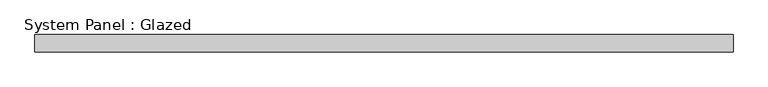
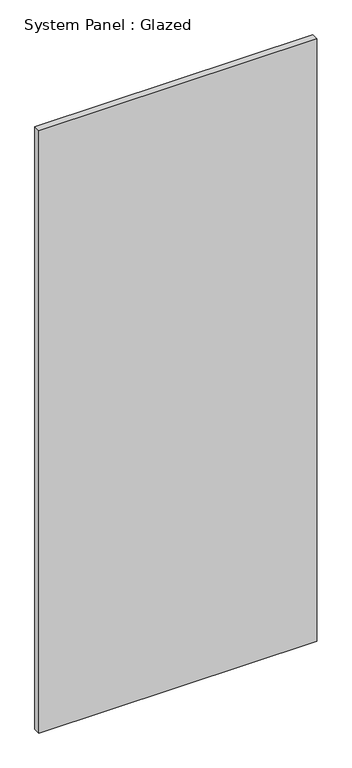
"""IFC4 building model written with IfcOpenShell, lengths in millimetres: plate geometry, System Panel : Glazed."""

from ifc_helpers import new_model, si_unit, origin, origin_with_axes, place, context, project, spatial, polyline, outline, extrude, source, transform, mapped, element, save


def system_panel_glazed_958d1135(model_context):
    return source(origin(), model_context, "Body", "SweptSolid", [
        extrude(outline(polyline([(511.175, 19.05), (-511.175, 19.05), (-511.175, 44.45), (511.175, 44.45), (511.175, 19.05)])), origin_with_axes(), (0.0, 0.0, 1.0), 2343.15),
    ])


if __name__ == "__main__":
    model = new_model("IFC4")
    model_context = context("Model", 3, world=origin())
    ifc_project = project(units=[si_unit("LENGTHUNIT", "METRE", prefix="MILLI")], contexts=[model_context])
    site = spatial("IfcSite", under=ifc_project)
    building = spatial("IfcBuilding", under=site)
    placement = place(None, origin())
    system_panel_glazed_shape = system_panel_glazed_958d1135(model_context)
    element("IfcPlate", 1, ObjectType="System Panel : Glazed", at=placement, inside=building, context=model_context, shape_type="MappedRepresentation", body=[
        mapped(system_panel_glazed_shape, transform((0.0, 0.0, 0.0), x_axis=(1.0, 0.0, 0.0), y_axis=(0.0, 1.0, 0.0), z_axis=(0.0, 0.0, 1.0))),
    ])
    save(model, "model.ifc")

# Revit data of these elements
# Type "System Panel : Glazed"
#   Construction Type Id = "GSP4R"
#   Analytic Construction = "1/8 in Pilkington single glazing"
#   Visual Light Transmittance = 0.9
#   Solar Heat Gain Coefficient = 0.86
#   Heat Transfer Coefficient (U) = 1.18115 BTU/(h·ft²·°F)
# Element 1 (IfcPlate, "System Panel : Glazed")
#   Materials on its faces: "Glass"
# Materials
#   "Glass": class "Glass", colour RGB 0 128 192, transparency 0.75, Description = "Soda Lime Glass", Cost = 0
